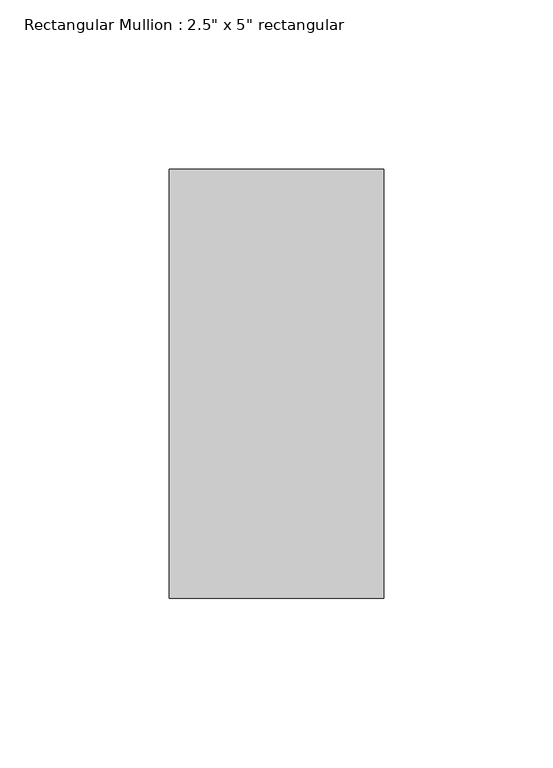
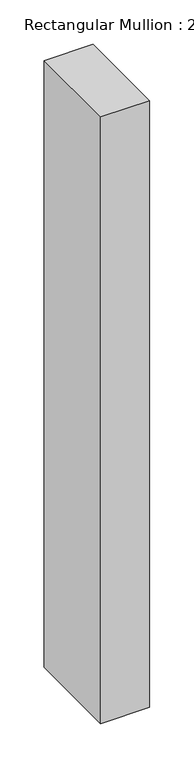
"""IFC4 building model written with IfcOpenShell, lengths in millimetres: member geometry."""

from ifc_helpers import new_model, si_unit, frame, origin, place, context, project, spatial, polyline, outline, extrude, source, transform, mapped, element, save


def member_24f36acb(model_context):
    return source(origin(), model_context, "Body", "SweptSolid", [
        extrude(outline(polyline([(0.0, 63.5), (0.0, -63.5), (-63.5, -63.5), (-63.5, 63.5), (0.0, 63.5)])), frame((0.0, 0.0, -832.5361093), z_axis=(0.0, 0.0, 1.0), x_axis=(1.0, 0.0, 0.0)), (0.0, 0.0, 1.0), 832.5361093),
    ])


if __name__ == "__main__":
    model = new_model("IFC4")
    model_context = context("Model", 3, world=origin())
    ifc_project = project(units=[si_unit("LENGTHUNIT", "METRE", prefix="MILLI")], contexts=[model_context])
    site = spatial("IfcSite", under=ifc_project)
    building = spatial("IfcBuilding", under=site)
    placement = place(None, origin())
    member_shape = member_24f36acb(model_context)
    element("IfcMember", 1, ObjectType="Rectangular Mullion : 2.5\" x 5\" rectangular", at=placement, inside=building, context=model_context, shape_type="MappedRepresentation", body=[
        mapped(member_shape, transform((0.0, 0.0, 0.0), x_axis=(1.0, 0.0, 0.0), y_axis=(0.0, 1.0, 0.0), z_axis=(0.0, 0.0, 1.0))),
    ])
    save(model, "model.ifc")

# Revit data of these elements
# Type "Rectangular Mullion : 2.5\" x 5\" rectangular"
#   built-in parameter 1007304 = 0.416667 (stored number, unit not read)
#   built-in parameter 1007301 = 0.104167 (stored number, unit not read)
#   built-in parameter 1007300 = 0.104167 (stored number, unit not read)
# Element 1 (IfcMember, "Rectangular Mullion : 2.5\" x 5\" rectangular")
#   Materials on its faces: "Aluminum"
# Materials
#   "Aluminum": class "Metal", colour RGB 247 247 247, transparency 0, Description = "Aluminum 6061", Cost = 0
